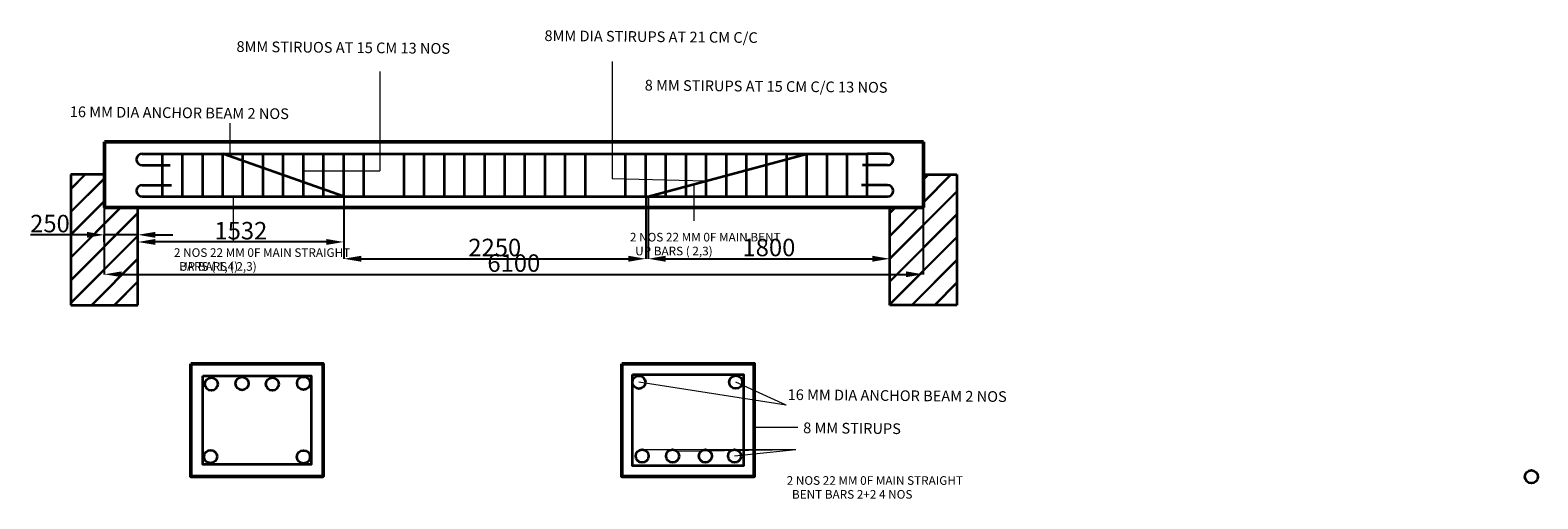
# Model space of a CAD drawing. Units: metres. Extents: x 702 to 11931, y -1477 to 2011.
import ezdxf

# ---------------------------------------------------------------- set-up
doc = ezdxf.new("R2010")
doc.units = ezdxf.units.M
for name, color, linetype, lineweight in [('A-WALL', 7, 'Continuous', 35), ('A-WALL-PATT', 8, 'Continuous', 18), ('S-ANNO-DIMS', 2, 'Continuous', 18), ('S-ANNO-TEXT', 3, 'Continuous', 18), ('S-BEAM', 7, 'Continuous', 50), ('S-REIN', 1, 'Continuous', 35)]:
    doc.layers.add(name, color=color, linetype=linetype, lineweight=lineweight)
doc.styles.get("Standard").update_dxf_attribs({"font": 'arial.ttf'})
doc.dimstyles.new('ISO-25', dxfattribs={"dimtxt": 130, "dimasz": 130, "dimexe": 1.25, "dimexo": 0.625, "dimtad": 1, "dimdec": 0, "dimtxsty": 'Standard', "dimcen": 2.5, "dimadec": 0, "dimazin": 0, "dimtfac": 1, "dimtdec": 0, "dimtmove": 0, "dimatfit": 3, "dimfxl": 1, "dimarcsym": 0})

# ---------------------------------------------------------------- blocks, each defined once
blk = doc.blocks.new('*D1')
at = {"layer": 'Defpoints', "color": 0, "transparency": 16777216}
for p in [(1254, 691), (7354, 691), (7354, 194)]:
    blk.add_point(p, dxfattribs=at)
at = {"layer": 'S-ANNO-DIMS', "color": 0, "lineweight": -2, "transparency": 16777216}
for p, q in [((1254, 690), (1254, 193)), ((7354, 690), (7354, 193)), ((1384, 194), (7224, 194))]:
    blk.add_line(p, q, dxfattribs=at)
at = {"layer": 'S-ANNO-DIMS', "color": 0, "transparency": 16777216}
for points in [[(1384, 216), (1384, 173), (1254, 194)], [(7224, 216), (7224, 173), (7354, 194)]]:
    blk.add_solid(points, dxfattribs=at)
at = {"layer": 'S-ANNO-DIMS', "color": 0, "transparency": 16777216, "insert": (4304, 261), "char_height": 130, "attachment_point": 5}
blk.add_mtext('6100', dxfattribs=at)
blk = doc.blocks.new('*D2')
at = {"layer": 'Defpoints', "color": 0, "transparency": 16777216}
for p in [(1504, 691), (3037, 772), (1504, 435)]:
    blk.add_point(p, dxfattribs=at)
at = {"layer": 'S-ANNO-DIMS', "color": 0, "lineweight": -2, "transparency": 16777216}
for p, q in [((1504, 690), (1504, 434)), ((3037, 771), (3037, 434)), ((2907, 435), (1634, 435))]:
    blk.add_line(p, q, dxfattribs=at)
at = {"layer": 'S-ANNO-DIMS', "color": 0, "transparency": 16777216}
for points in [[(1634, 457), (1634, 413), (1504, 435)], [(2907, 457), (2907, 413), (3037, 435)]]:
    blk.add_solid(points, dxfattribs=at)
at = {"layer": 'S-ANNO-DIMS', "color": 0, "transparency": 16777216, "insert": (2271, 502), "char_height": 130, "attachment_point": 5}
blk.add_mtext('1532', dxfattribs=at)
blk = doc.blocks.new('*D3')
at = {"layer": 'Defpoints', "color": 0, "transparency": 16777216}
for p in [(1254, 488), (1254, 435), (1504, 435)]:
    blk.add_point(p, dxfattribs=at)
at = {"layer": 'S-ANNO-DIMS', "color": 0, "lineweight": -2, "transparency": 16777216}
for p, q in [((1124, 488), (704, 488)), ((1254, 436), (1254, 489)), ((1504, 488), (1254, 488)), ((1504, 436), (1504, 489)), ((1634, 488), (1764, 488))]:
    blk.add_line(p, q, dxfattribs=at)
at = {"layer": 'S-ANNO-DIMS', "color": 0, "transparency": 16777216}
for points in [[(1124, 510), (1124, 466), (1254, 488)], [(1634, 510), (1634, 466), (1504, 488)]]:
    blk.add_solid(points, dxfattribs=at)
at = {"layer": 'S-ANNO-DIMS', "color": 0, "transparency": 16777216, "insert": (849, 555), "char_height": 130, "attachment_point": 5}
blk.add_mtext('250', dxfattribs=at)
blk = doc.blocks.new('*D4')
at = {"layer": 'Defpoints', "color": 0, "transparency": 16777216}
for p in [(5304, 772), (7104, 691), (7104, 310)]:
    blk.add_point(p, dxfattribs=at)
at = {"layer": 'S-ANNO-DIMS', "color": 0, "lineweight": -2, "transparency": 16777216}
for p, q in [((5304, 771), (5304, 309)), ((7104, 690), (7104, 309)), ((5434, 310), (6974, 310))]:
    blk.add_line(p, q, dxfattribs=at)
at = {"layer": 'S-ANNO-DIMS', "color": 0, "transparency": 16777216}
for points in [[(5434, 332), (5434, 288), (5304, 310)], [(6974, 332), (6974, 288), (7104, 310)]]:
    blk.add_solid(points, dxfattribs=at)
at = {"layer": 'S-ANNO-DIMS', "color": 0, "transparency": 16777216, "insert": (6204, 377), "char_height": 130, "attachment_point": 5}
blk.add_mtext('1800', dxfattribs=at)
blk = doc.blocks.new('*D5')
at = {"layer": 'Defpoints', "color": 0, "transparency": 16777216}
for p in [(3037, 772), (5287, 772), (5287, 310)]:
    blk.add_point(p, dxfattribs=at)
at = {"layer": 'S-ANNO-DIMS', "color": 0, "lineweight": -2, "transparency": 16777216}
for p, q in [((3037, 771), (3037, 309)), ((5287, 771), (5287, 309)), ((3167, 310), (5157, 310))]:
    blk.add_line(p, q, dxfattribs=at)
at = {"layer": 'S-ANNO-DIMS', "color": 0, "transparency": 16777216}
for points in [[(3167, 332), (3167, 288), (3037, 310)], [(5157, 332), (5157, 288), (5287, 310)]]:
    blk.add_solid(points, dxfattribs=at)
at = {"layer": 'S-ANNO-DIMS', "color": 0, "transparency": 16777216, "insert": (4162, 377), "char_height": 130, "attachment_point": 5}
blk.add_mtext('2250', dxfattribs=at)

msp = doc.modelspace()

# ---------------------------------------------------------------- hatches: boundary and pattern name
at = {"layer": 'A-WALL-PATT'}
h = msp.add_hatch(dxfattribs=at)
h.set_pattern_fill('JIS_RC_15', color=256, scale=8)
h.paths.add_polyline_path([(1504.3, 691.1), (1254.3, 691.1), (1254.3, 936.1), (1004.3, 936.1), (1004.3, -34.6), (1504.3, -34.6)])
h.paths.add_polyline_path([(7604.3, 936.1), (7354.3, 936.1), (7354.3, 691.1), (7104.3, 691.1), (7104.3, -34.9), (7604.3, -34.9)])

# ---------------------------------------------------------------- linework, layer by layer
at = {"layer": 'A-WALL'}
for p, q in [((1254.3, 936.1), (1004.3, 936.1)), ((1004.3, 936.1), (1004.3, -34.6)), ((7354.3, 936.1), (7604.3, 936.1)), ((7604.3, 936.1), (7604.3, -34.9)), ((1504.3, -34.6), (1504.3, 691.1)), ((7104.3, -34.9), (7104.3, 691.1)), ((1004.3, -34.6), (1504.3, -34.6)), ((7604.3, -34.9), (7104.3, -34.9))]:
    msp.add_line(p, q, dxfattribs=at)
at = {"layer": 'S-ANNO-TEXT'}
for p, q in [((3306.1, 1703), (3306.1, 965)), ((5035.5, 1778.8), (5035.5, 907.1)), ((2189.7, 1318.7), (2189.7, 1092)), ((2736.8, 965), (3306.1, 965)), ((5035.5, 907.1), (5736.8, 889.1)), ((5647.4, 593.4), (5647.4, 864.9)), ((2216.9, 436.9), (2216.9, 772.1)), ((6332.7, -780.2), (5236.1, -608.8)), ((6332.7, -780.2), (5957.5, -608.3)), ((6418.7, -945.6), (6094.4, -945.1)), ((6404.5, -1111.4), (5248, -1111.4)), ((6404.5, -1111.4), (5521, -1124.4)), ((6404.5, -1111.4), (5775.6, -1120.7)), ((6404.5, -1111.4), (5948.3, -1158.3))]:
    msp.add_line(p, q, dxfattribs=at)
at = {"layer": 'S-BEAM'}
for p, q in [((1254.3, 691.1), (1254.3, 1181.1)), ((1254.3, 1181.1), (7354.3, 1181.1)), ((7354.3, 1181.1), (7354.3, 691.1)), ((1254.3, 691.1), (7354.3, 691.1))]:
    msp.add_line(p, q, dxfattribs=at)
for points in [[(1897.6, -471.9), (2883.8, -471.9), (2883.8, -1310.4), (1897.6, -1310.4)], [(5108.2, -471.9), (6094.4, -471.9), (6094.4, -1310.4), (5108.2, -1310.4)]]:
    msp.add_lwpolyline(points, close=True, dxfattribs=at)
at = {"layer": 'S-REIN'}
for p, q in [((1536.8, 1092), (6936.8, 1092)), ((1686.8, 772.1), (1686.8, 1092)), ((1836.8, 772.1), (1836.8, 1092)), ((1986.8, 772.1), (1986.8, 1092)), ((2136.8, 772.1), (2136.8, 1092)), ((3036.8, 772.1), (2136.8, 1092)), ((2286.8, 772.1), (2286.8, 1092)), ((2436.8, 772.1), (2436.8, 1092)), ((2586.8, 772.1), (2586.8, 1092)), ((2736.8, 772.1), (2736.8, 1092)), ((2886.8, 772.1), (2886.8, 1092)), ((3036.8, 772.1), (3036.8, 1092)), ((3186.8, 772.1), (3186.8, 1092)), ((3486.8, 772.1), (3486.8, 1092)), ((3636.8, 772.1), (3636.8, 1092)), ((3786.8, 772.1), (3786.8, 1092)), ((3936.8, 772.1), (3936.8, 1092)), ((4086.8, 772.1), (4086.8, 1092)), ((4236.8, 772.1), (4236.8, 1092)), ((4386.8, 772.1), (4386.8, 1092)), ((4536.8, 772.1), (4536.8, 1092)), ((4686.8, 772.1), (4686.8, 1092)), ((4836.8, 772.1), (4836.8, 1092)), ((5136.8, 772.1), (5136.8, 1092)), ((5286.8, 772.1), (5286.8, 1092)), ((5304.3, 772.1), (6486.8, 1092)), ((5436.8, 772.1), (5436.8, 1092)), ((5586.8, 772.1), (5586.8, 1092)), ((5736.8, 772.1), (5736.8, 1092)), ((5886.8, 772.1), (5886.8, 1092)), ((6036.8, 772.1), (6036.8, 1092)), ((6186.8, 772.1), (6186.8, 1092)), ((6336.8, 772.1), (6336.8, 1092)), ((6486.8, 772.1), (6486.8, 1092)), ((6636.8, 772.1), (6636.8, 1092)), ((6786.8, 772.1), (6786.8, 1092)), ((6936.8, 772.1), (6936.8, 1092)), ((7086.8, 1092), (6936.8, 1092)), ((1536.8, 1005.6), (1744.9, 1005.6)), ((7086.8, 1006), (6900.4, 1006)), ((1536.8, 858.1), (1754.7, 858.1)), ((7086.8, 858.1), (6893.8, 858.1)), ((1536.8, 772.1), (6936.8, 772.1)), ((6936.8, 772.1), (7086.8, 772.1)), ((7086.8, 772.1), (7086.8, 772.1))]:
    msp.add_line(p, q, dxfattribs=at)
for points in [[(5187.2, -551), (6015.4, -551), (6015.4, -1231.4), (5187.2, -1231.4)], [(1987.2, -561.6), (2794.2, -561.6), (2794.2, -1220.7), (1987.2, -1220.7)]]:
    msp.add_lwpolyline(points, close=True, dxfattribs=at)
for centre in [(5236.1, -608.8), (5957.5, -608.3), (2051, -622.8), (2279.8, -618.4), (2505.3, -622.8), (2737.6, -616), (2045, -1162.7), (2737.2, -1164.4), (5259.9, -1158.3), (5486.5, -1158.3), (5730.5, -1158.3), (5948.3, -1158.3), (11882.7, -1312.6)]:
    msp.add_circle(centre, 48.4, dxfattribs=at)
for centre, radius, start, end in [((1536.8, 1048.8), 43.2, 90, 270), ((7086.8, 1049), 43, 270, 90), ((1536.8, 815.1), 43, 90, 270), ((7086.8, 815.1), 43, 270, 90)]:
    msp.add_arc(centre, radius, start, end, dxfattribs=at)

# ---------------------------------------------------------------- texts
at = {"layer": 'S-ANNO-TEXT'}
for s, p in [('8MM STIRUOS AT 15 CM 13 NOS', (2237.9, 1849.6)), ('8MM DIA STIRUPS AT 21 CM C/C  ', (4531.9, 1930.5)), ('8 MM STIRUPS AT 15 CM C/C 13 NOS', (5278.6, 1562)), ('16 MM DIA ANCHOR BEAM 2 NOS', (996.5, 1364.3)), ('16 MM DIA ANCHOR BEAM 2 NOS', (6343.1, -740.8)), ('8 MM STIRUPS ', (6458.7, -988.1))]:
    msp.add_text(s, height=79.62, rotation=359.46604, dxfattribs=at).set_placement(p)
for s, p in [('2 NOS 22 MM 0F MAIN BENT', (5168.7, 438.5)), ('2 NOS 22 MM 0F MAIN STRAIGHT', (1772.5, 323.7)), ('2 NOS 22 MM 0F MAIN ', (1772.5, 323.7)), ('  UP BARS ( 2,3)', (5168.7, 335.3)), ('  UP BARS ( 2,3)', (1772.5, 220.6)), ('  BARS ( 1,4)', (1772.5, 220.6)), ('2 NOS 22 MM 0F MAIN STRAIGHT', (6336.4, -1372.4)), ('  BENT BARS 2+2 4 NOS', (6336.4, -1475.5))]:
    msp.add_text(s, height=64.215, dxfattribs=at).set_placement(p)
at = {"layer": 'S-ANNO-TEXT', "insert": (1235.9, 1442.6), "char_height": 0.0803, "attachment_point": 1}
msp.add_mtext_dynamic_manual_height_columns('16MM DIA ANCHOR BEAM 2 NOS ', width=23.847, gutter_width=0.402, heights=[0], dxfattribs=at)

# ---------------------------------------------------------------- dimensions: what is measured, and where the dimension line sits
at = {"layer": 'S-ANNO-DIMS'}
for base, p1, p2, picture, middle in [((7354.3, 194.5), (1254.3, 691.1), (7354.3, 691.1), '*D1', (4304.3, 261.5)), ((1504.2721, 435.0778), (3036.7673, 772.1217), (1504.2721, 691.1217), '*D2', (2270.5197, 502.1216)), ((5286.8, 309.9), (3036.8, 772.1), (5286.8, 772.1), '*D5', (4161.8, 376.9)), ((7104.3, 309.9), (5304.3, 772.1), (7104.3, 691.1), '*D4', (6204.3, 376.9)), ((1254.3, 487.9), (1504.3, 435.1), (1254.3, 435.1), '*D3', (849.1, 554.9))]:
    dim = msp.add_linear_dim(base=base, p1=p1, p2=p2, dimstyle='ISO-25', override={"dimclrd": 0, "dimclre": 0, "dimclrt": 0}, dxfattribs=at)
    dim.commit()
    dim.dimension.update_dxf_attribs({"geometry": picture, "text_midpoint": middle})

doc.saveas('drawing.dxf')
